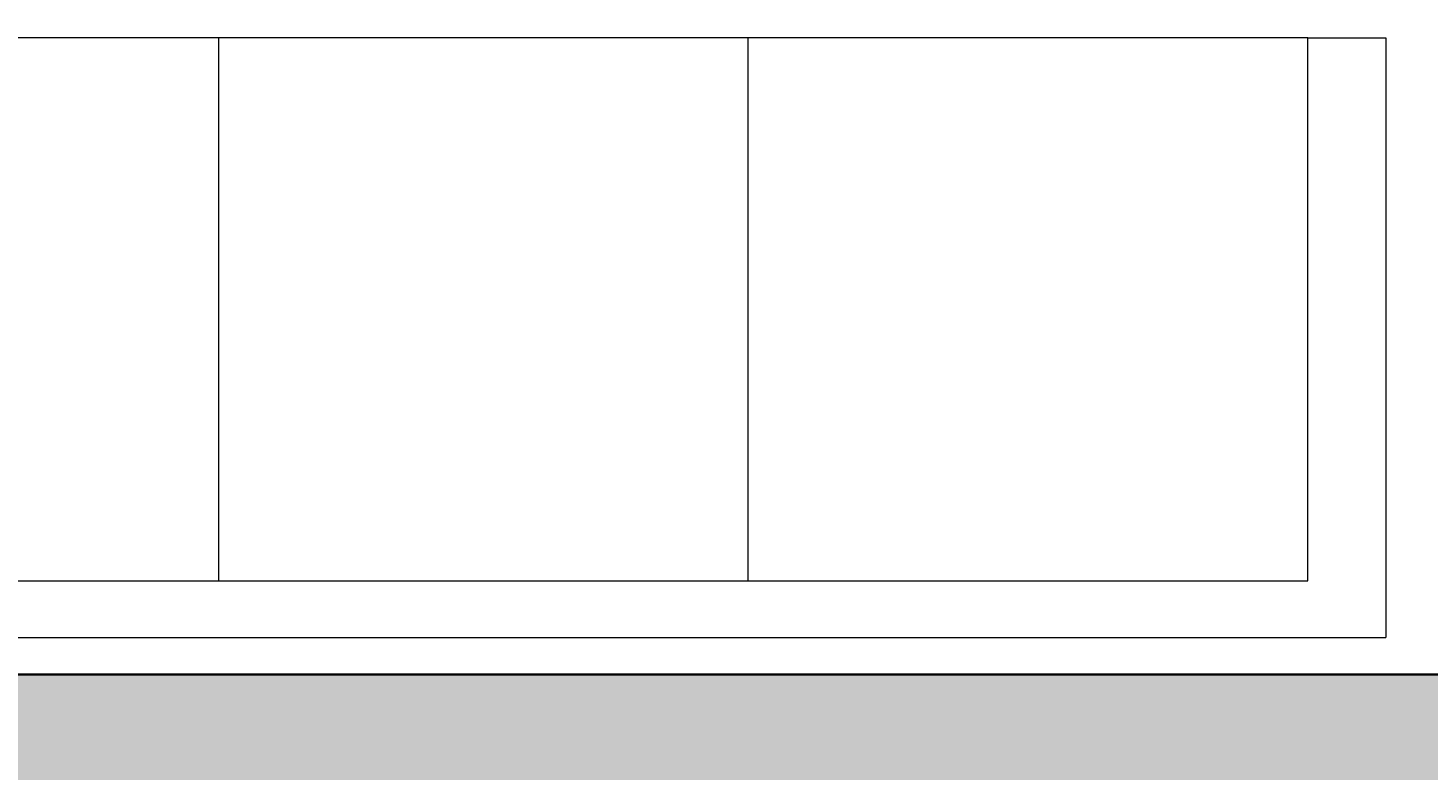
# Model space of a CAD drawing. Units: inches. Extents: x 1998 to 2588, y 1139 to 1977.
# Tile 126 of 134: x 2429 to 2489, y 1637 to 1669. Entities that reach past the tile are written whole.
import ezdxf

# ---------------------------------------------------------------- set-up
doc = ezdxf.new("R2010")
doc.units = ezdxf.units.IN
for name, color, linetype, lineweight in [('A-ANNO-DIMS', 2, 'Continuous', 18), ('A-WALL-PATT', 252, 'Continuous', 13), ('FUR', 21, 'Continuous', 18), ('WALL', 200, 'Continuous', 35)]:
    doc.layers.add(name, color=color, linetype=linetype, lineweight=lineweight)
doc.styles.get("Standard").update_dxf_attribs({"font": 'arial.ttf'})
doc.dimstyles.get("Standard").update_dxf_attribs({"dimtxt": 0.18, "dimasz": 0.18, "dimexe": 0.18, "dimexo": 0.0625, "dimgap": 0.09, "dimtad": 0, "dimtih": 1, "dimtoh": 1, "dimdec": 4, "dimzin": 0, "dimdsep": 46, "dimtxsty": 'Standard', "dimcen": 0.09, "dimadec": 0, "dimazin": 0, "dimtfac": 1, "dimtdec": 4, "dimtofl": 0, "dimtmove": 0, "dimatfit": 3, "dimfxl": 1, "dimtolj": 1, "dimtzin": 0, "dimarcsym": 0})

# ---------------------------------------------------------------- blocks, each defined once
blk = doc.blocks.new('SOFA-THREE-SEAT')
for p, q in [((24.453, 25.615), (24.453, 2.416)), ((47.077, 25.615), (47.077, 2.416)), ((71.008, 25.615), (74.336, 25.615)), ((74.336, 25.615), (74.336, 0)), ((0, 0), (74.336, 0))]:
    blk.add_line(p, q)
blk.add_lwpolyline([(3.604, 2.416), (71.008, 2.416), (71.008, 25.615), (3.604, 25.615)], close=True)
blk = doc.blocks.new('*D24')
at = {"layer": 'A-ANNO-DIMS', "color": 0, "lineweight": -2, "transparency": 16777216}
for p, q in [((2398.535, 1911.232), (2588.309, 1911.232)), ((2588.129, 1911.052), (2588.129, 1570.164)), ((2588.129, 1228.912), (2588.129, 1569.8)), ((2527.535, 1228.732), (2588.309, 1228.732))]:
    blk.add_line(p, q, dxfattribs=at)
at = {"layer": 'A-ANNO-DIMS', "color": 0, "transparency": 16777216}
for points in [[(2588.099, 1911.052), (2588.159, 1911.052), (2588.129, 1911.232)], [(2588.099, 1228.912), (2588.159, 1228.912), (2588.129, 1228.732)]]:
    blk.add_solid(points, dxfattribs=at)
at = {"layer": 'Defpoints', "color": 0, "transparency": 16777216}
for p in [(2398.473, 1911.232), (2588.129, 1911.232), (2527.473, 1228.732)]:
    blk.add_point(p, dxfattribs=at)
at = {"layer": 'A-ANNO-DIMS', "color": 0, "transparency": 16777216, "insert": (2588.129, 1569.982), "char_height": 0.18, "attachment_point": 5}
blk.add_mtext('\\A1;682.5', dxfattribs=at)

msp = doc.modelspace()

# ---------------------------------------------------------------- hatches: boundary and pattern name
at = {"layer": 'A-WALL-PATT'}
h = msp.add_hatch(color=256, dxfattribs=at)
h.dxf.hatch_style = 1
h.paths.add_polyline_path([(2527.4729, 1362.2324), (2510.9729, 1362.2324), (2510.9729, 1357.7324), (2518.4729, 1357.7324), (2518.4729, 1237.7324), (2503.1458, 1237.7324), (2503.1458, 1228.7324), (2527.4729, 1228.7324)])
h.paths.add_polyline_path([(2490.5682, 1362.2324), (2398.4729, 1362.2324), (2398.4729, 1357.7324), (2490.5682, 1357.7324)])
h.paths.add_polyline_path([(2224.9729, 1264.7324), (2222.9729, 1264.7324), (2222.9729, 1232.4125), (2341.4729, 1232.4125), (2341.4729, 1234.4125), (2224.9729, 1234.4125)])
h.paths.add_polyline_path([(2334.5332, 1273.7324), (2264.7638, 1273.7324), (2264.7638, 1269.5611, -0.043659), (2264.3413, 1264.7324), (2334.5332, 1264.7324)])
h.paths.add_polyline_path([(2236.9551, 1273.7324), (2234.4125, 1273.7324), (2234.4125, 1264.7324), (2236.9551, 1264.7324), (2236.9551, 1269.5611)])
h.paths.add_polyline_path([(2222.9729, 1293.2324), (2096.9729, 1293.2324), (2096.9729, 1345.0966), (2087.9729, 1345.0966), (2087.9729, 1284.2324), (2222.9729, 1284.2324), (2222.9729, 1285.137)])
h.paths.add_polyline_path([(2096.9729, 1458.7927), (2087.9729, 1458.7927), (2087.9729, 1417.7324), (2087.9729, 1413.2324), (2096.9729, 1413.2324), (2096.9729, 1417.7324)])
h.paths.add_polyline_path([(2096.9729, 1413.2324), (2087.9729, 1413.2324), (2087.9729, 1365.5012), (2096.9729, 1365.5012), (2096.9729, 1369.3358)])
h.paths.add_polyline_path([(2186.2943, 1417.7324), (2138.6074, 1417.7324), (2096.9729, 1417.7324), (2096.9729, 1413.2324), (2138.6074, 1413.2324), (2186.2943, 1413.2324)])
h.paths.add_polyline_path([(2181.4729, 1465.7324), (2176.9729, 1465.7324), (2176.9729, 1451.6434), (2181.4729, 1451.6434)])
h.paths.add_polyline_path([(2181.4729, 1422.1664), (2176.9729, 1422.1664), (2176.9729, 1417.7324), (2181.4729, 1417.7324)])
h.paths.add_polyline_path([(2063.9729, 1465.7324), (2087.9729, 1465.7324), (2087.9729, 1470.2324), (2059.4729, 1470.2324), (2059.4729, 1413.2324), (2087.9729, 1413.2324), (2087.9729, 1417.7324), (2063.9729, 1417.7324)])
h.paths.add_polyline_path([(2181.4729, 1755.2324), (2176.9729, 1755.2324), (2176.9729, 1748.6798), (2177.0513, 1748.6798), (2181.4729, 1748.6798)])
h.paths.add_polyline_path([(2227.4729, 1707.2324), (2220.4647, 1707.2324), (2220.4647, 1702.7324), (2222.9729, 1702.7324), (2222.9729, 1604.637), (2227.4729, 1604.637)])
h.paths.add_polyline_path([(2114.9729, 1702.7324), (2105.9729, 1702.7324), (2105.9729, 1628.4781, -0.0318759), (2110.1012, 1628.7416), (2114.9729, 1628.7416)])
h.paths.add_polyline_path([(2345.9729, 1739.3278), (2341.4729, 1739.3278), (2341.4729, 1647.5211), (2345.9729, 1647.5211)])
h.paths.add_polyline_path([(2350.6273, 1641.2324), (2345.9729, 1641.2324), (2345.9729, 1636.7324), (2350.6273, 1636.7324), (2350.6273, 1639.8729)])
h.paths.add_polyline_path([(2501.9729, 1641.2324), (2407.9729, 1641.2324), (2392.5005, 1641.2324), (2392.5005, 1639.8729), (2392.5005, 1636.7324), (2501.9729, 1636.7324)])
h.paths.add_polyline_path([(2510.9729, 1755.2324), (2501.9729, 1755.2324), (2501.9729, 1641.2324), (2510.9729, 1641.2324)])
h.paths.add_polyline_path([(2549.1786, 1641.2324), (2522.3775, 1641.2324), (2522.3775, 1636.7324), (2540.1786, 1636.7324), (2540.1786, 1480.7324), (2522.3775, 1480.7324), (2522.3775, 1476.2324), (2549.1786, 1476.2324)])
h.paths.add_polyline_path([(2498.1786, 1594.7324), (2407.9729, 1594.7324), (2407.9729, 1585.7324), (2416.9729, 1585.7324), (2489.1786, 1585.7324), (2489.1786, 1531.7324), (2416.9729, 1531.7324), (2407.9729, 1531.7324), (2407.9729, 1522.7324), (2498.1786, 1522.7324)])
h.paths.add_polyline_path([(2351.6437, 1480.7324), (2345.9729, 1480.7324), (2345.9729, 1476.2324), (2351.6437, 1476.2324), (2351.6437, 1477.5919)])
h.paths.add_polyline_path([(2501.9729, 1480.7324), (2498.1786, 1480.7324), (2407.9729, 1480.7324), (2393.5168, 1480.7324), (2393.5168, 1477.5919), (2393.5168, 1476.2324), (2501.9729, 1476.2324)])

# ---------------------------------------------------------------- linework, layer by layer
at = {"layer": 'WALL'}
for p, q in [((2501.9729, 1641.2324), (2391.5845, 1641.2324)), ((2407.9729, 1641.2324), (2549.1786, 1641.2324))]:
    msp.add_line(p, q, dxfattribs=at)

# ---------------------------------------------------------------- block references
at = {"layer": 'FUR'}
msp.add_blockref('SOFA-THREE-SEAT', (2412.6207, 1642.8172), dxfattribs=at)

# ---------------------------------------------------------------- dimensions: what is measured, and where the dimension line sits
at = {"layer": 'A-ANNO-DIMS'}
dim = msp.add_linear_dim(base=(2588.1286, 1911.2324), p1=(2527.4729, 1228.7324), p2=(2398.4729, 1911.2324), angle=90, dimstyle='Standard', override={"dimdec": 1, "dimlfac": 1, "dimrnd": 0, "dimzin": 0, "dimdsep": 46, "dimlunit": 2}, dxfattribs=at)
dim.commit()
dim.dimension.update_dxf_attribs({"geometry": '*D24', "text_midpoint": (2588.1286, 1569.9824)})

doc.saveas('drawing.dxf')
